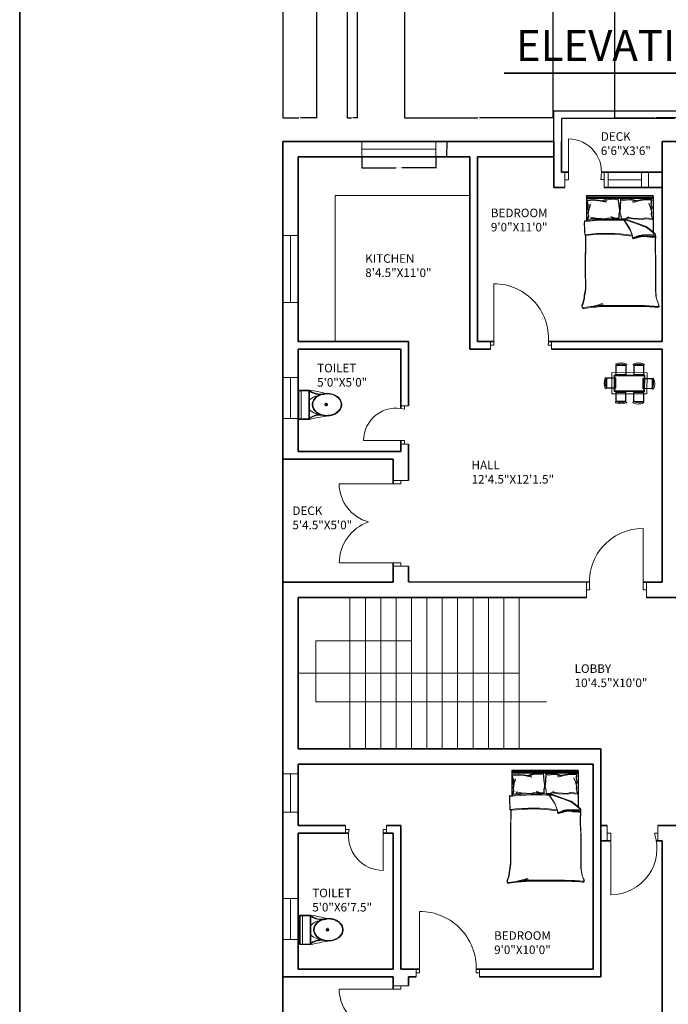
# Model space of a CAD drawing. Units: inches. Extents: x 2250 to 3629, y 982 to 2740.
# Tile 3 of 12: x 2250 to 2629, y 1543 to 2119. Entities that reach past the tile are written whole.
import ezdxf

# ---------------------------------------------------------------- set-up
doc = ezdxf.new("R2010")
doc.units = ezdxf.units.IN
for name, color, linetype, lineweight in [('A-ANNO-DIMS', 2, 'Continuous', 18), ('A-ANNO-TITL', 7, 'Continuous', 35), ('A-ANNO-TTLB', 7, 'Continuous', 35), ('A-AREA-IDEN', 7, 'Continuous', 18), ('A-DOOR', 3, 'Continuous', 18), ('A-FLOR-DECK', 7, 'Continuous', 25), ('A-FLOR-FIXT', 9, 'Continuous', 18), ('A-FLOR-STRS', 7, 'Continuous', 18), ('A-FURN', 8, 'Continuous', 13), ('A-GLAZ', 4, 'Continuous', 18), ('A-WALL', 7, 'Continuous', 35)]:
    doc.layers.add(name, color=color, linetype=linetype, lineweight=lineweight)
doc.styles.get("Standard").update_dxf_attribs({"font": 'arial.ttf'})
doc.dimstyles.get("Standard").update_dxf_attribs({"dimtxt": 0.18, "dimasz": 0.18, "dimexe": 0.18, "dimexo": 0.0625, "dimgap": 0.09, "dimtad": 0, "dimtih": 1, "dimtoh": 1, "dimdec": 4, "dimzin": 0, "dimdsep": 46, "dimtxsty": 'Standard', "dimcen": 0.09, "dimadec": 0, "dimazin": 0, "dimtfac": 1, "dimtdec": 4, "dimtofl": 0, "dimtmove": 0, "dimatfit": 3, "dimfxl": 1, "dimtolj": 1, "dimtzin": 0, "dimarcsym": 0})

# ---------------------------------------------------------------- blocks, each defined once
blk = doc.blocks.new('A$C31115884')
for p, q in [((258, 466), (258, 523)), ((283, 498), (223, 498)), ((0, 200), (0, 0)), ((520, 200), (0, 200)), ((10, 190), (10, 10)), ((510, 190), (10, 190)), ((510, 10), (510, 190)), ((520, 0), (520, 200)), ((510, 54), (0, 54)), ((10, 10), (510, 10)), ((0, 0), (520, 0))]:
    blk.add_line(p, q)
blk.add_circle((256, 496), 23.6)
for centre, radius, start, end in [((2778, -205), 2807, 165.4549, 171.7133), ((-295, 403), 365, 324.2091, 9.3499), ((-295, 403), 375, 324.2091, 9.3499), ((384, 406), 293, 190.2774, 224.1564), ((139, 406), 293, 315.8436, 2.6563), ((806, 403), 375, 179.2036, 215.7909), ((806, 403), 365, 170.6501, 215.7909), ((3237, 905), 2807, 188.2867, 194.5451)]:
    blk.add_arc(centre, radius, start, end)
blk.add_ellipse((256, 510), major_axis=(0, -261), ratio=0.772727)
blk.add_open_spline([(256, 259), (263, 259), (270, 260), (288, 262), (299, 265), (320, 273), (330, 278), (350, 291), (360, 299), (378, 316), (386, 326), (402, 347), (409, 358), (421, 383), (427, 395), (436, 422), (440, 436), (445, 465), (447, 480), (448, 509), (448, 524), (445, 553), (443, 568), (436, 596), (432, 610), (422, 636), (416, 649), (402, 672), (395, 683), (379, 703), (370, 712), (351, 728), (341, 735), (321, 746), (310, 751), (289, 757), (278, 759), (256, 761), (245, 761), (223, 757), (212, 754), (191, 746), (181, 741), (161, 728), (151, 720), (133, 703), (125, 693), (110, 672), (103, 660), (90, 636), (85, 623), (76, 596), (72, 582), (67, 553), (66, 538), (64, 509), (65, 494), (68, 465), (70, 450), (77, 422), (81, 408), (91, 382), (97, 370), (111, 346), (118, 335), (135, 316), (144, 307), (162, 291), (172, 284), (193, 273), (203, 269), (225, 262), (236, 260), (250, 259), (253, 259), (256, 259)], degree=3, knots=[0, 0, 0, 0, 0.110105, 0.110105, 0.285049, 0.285049, 0.459994, 0.459994, 0.634938, 0.634938, 0.809882, 0.809882, 0.984827, 0.984827, 1.159771, 1.159771, 1.334715, 1.334715, 1.50966, 1.50966, 1.684604, 1.684604, 1.859549, 1.859549, 2.034493, 2.034493, 2.209437, 2.209437, 2.384382, 2.384382, 2.559326, 2.559326, 2.73427, 2.73427, 2.909215, 2.909215, 3.084159, 3.084159, 3.259103, 3.259103, 3.434048, 3.434048, 3.608992, 3.608992, 3.783936, 3.783936, 3.958881, 3.958881, 4.133825, 4.133825, 4.30877, 4.30877, 4.483714, 4.483714, 4.658658, 4.658658, 4.833603, 4.833603, 5.008547, 5.008547, 5.183491, 5.183491, 5.358436, 5.358436, 5.53338, 5.53338, 5.708324, 5.708324, 5.883269, 5.883269, 6.058213, 6.058213, 6.233158, 6.233158, 6.283185, 6.283185, 6.283185, 6.283185])
blk = doc.blocks.new('DR-36-BED-NW')
for p, q in [((2, 2.25), (2, 38.25)), ((0, 4.5), (0, 0)), ((0, 0), (0, 2.25)), ((0, 2.25), (2, 2.25)), ((35.76, 2.25), (33.76, 2.25)), ((35.76, 4.5), (35.76, 0)), ((35.76, 0), (35.76, 2.25))]:
    blk.add_line(p, q)
blk.add_arc((2, 6.24), 32.01, 352.83756, 90)
blk = doc.blocks.new('DR-24-DECK-NW')
for p, q in [((2, 4.5), (2, 28.5)), ((0, 9), (0, 0)), ((22.88, 0), (22.88, 9)), ((22.88, 9), (22.88, 4.79)), ((0, 0), (0, 4.5)), ((0, 4.5), (2, 4.5)), ((22.88, 4.79), (20.88, 4.79))]:
    blk.add_line(p, q)
blk.add_arc((2, 9.13), 19.37, 347.05433, 90)
blk = doc.blocks.new('DR-72-DECK-WEST-N')
for p, q in [((36, 48.33), (0, 48.33)), ((31.5, 50.33), (40.5, 50.33)), ((40.5, 50.33), (36, 50.33)), ((36, 50.33), (36, 48.33)), ((36, 2), (0, 2)), ((36, 0), (36, 2)), ((31.5, 0), (40.5, 0)), ((40.5, 0), (36, 0))]:
    blk.add_line(p, q)
for centre, radius, start, end in [((23.09, 48.33), 23.09, 180, 255.18417), ((25.75, 1.72), 25.76, 109.42773, 179.37341)]:
    blk.add_arc(centre, radius, start, end)
blk = doc.blocks.new('DR-24-BATH-NW')
for p, q in [((21.75, 22.45), (26.25, 22.45)), ((26.25, 22.45), (24, 22.45)), ((24, 22.45), (24, 20.45)), ((24, 2), (0, 2)), ((24, 0), (24, 2)), ((21.75, 0), (26.25, 0)), ((26.25, 0), (24, 0))]:
    blk.add_line(p, q)
blk.add_arc((19.09, 2), 19.09, 75.08916, 180)
blk = doc.blocks.new('DR-72-DECK-WEST-S')
for p, q in [((31.5, 47.46), (40.5, 47.46)), ((40.5, 47.46), (36, 47.46)), ((36, 47.46), (36, 45.46)), ((36, 45.46), (0, 45.46)), ((36, 2), (0, 2)), ((36, 0), (36, 2)), ((31.5, 0), (40.5, 0)), ((40.5, 0), (36, 0))]:
    blk.add_line(p, q)
for centre, radius, start, end in [((22.88, 45.46), 22.88, 180, 254.62165), ((25.61, -0.82), 25.77, 109.96423, 173.71154)]:
    blk.add_arc(centre, radius, start, end)
blk = doc.blocks.new('DR-24-BATH-WEST')
for p, q in [((0, 26.25), (0, 21.75)), ((0, 21.75), (0, 24)), ((0, 24), (2, 24)), ((23.91, 24), (21.91, 24)), ((21.91, 24), (21.91, 0)), ((23.91, 21.75), (23.91, 26.25)), ((23.91, 26.25), (23.91, 24))]:
    blk.add_line(p, q)
blk.add_arc((21.91, 20.26), 20.25, 169.34509, 270)
blk = doc.blocks.new('DR-36-BED-WEST')
for p, q in [((2, 2.25), (2, 38.25)), ((0, 4.5), (0, 0)), ((0, 0), (0, 2.25)), ((0, 2.25), (2, 2.25)), ((37.11, 2.25), (35.11, 2.25)), ((37.11, 4.5), (37.11, 0)), ((37.11, 0), (37.11, 2.25))]:
    blk.add_line(p, q)
blk.add_arc((2, 5.02), 33.23, 355.21404, 90)
blk = doc.blocks.new('DR-36-ENTRY-SW')
for p, q in [((0, 40.5), (0, 31.5)), ((29.54, 31.5), (29.54, 40.5)), ((0, 31.5), (0, 36)), ((0, 36), (2, 36)), ((2, 36), (2, 0)), ((29.54, 36), (27.54, 36))]:
    blk.add_line(p, q)
blk.add_arc((2, 27.06), 27.06, 270, 19.28442)
blk = doc.blocks.new('DR-36-ENTRY-NW')
for p, q in [((33.05, 4.5), (33.05, 40.5)), ((0, 9.04), (0, 0)), ((35.05, 9.01), (35.05, 0)), ((0, 0), (0, 4.52)), ((0, 4.52), (2, 4.52)), ((35.05, 4.5), (33.05, 4.5)), ((35.05, 0), (35.05, 4.5))]:
    blk.add_line(p, q)
blk.add_arc((33.05, 9.12), 31.39, 90, 188.41497)
blk = doc.blocks.new('WIN-DECK-NW')
for p, q in [((0.07, 4.5), (0.07, 9)), ((0.07, 9), (0.07, 1.12)), ((19.52, 9), (19.52, 0)), ((0.07, 1.12), (0, 0)), ((19.52, 4.5), (0.07, 4.5)), ((19.52, 0), (19.52, 4.5))]:
    blk.add_line(p, q)
blk = doc.blocks.new('WIN-KITCHEN-NW-A')
for p, q in [((0, 9), (0, 0)), ((43.24, 4.5), (43.24, 9)), ((43.24, 9), (43.24, 0)), ((0, 4.5), (43.24, 4.5))]:
    blk.add_line(p, q)
blk = doc.blocks.new('WIN-KITCHEN-NW-B')
for p, q in [((0, 39.2), (9, 39.2)), ((4.5, 0), (4.5, 39.2)), ((9, 0), (0, 0)), ((0, 0), (4.5, 0))]:
    blk.add_line(p, q)
blk = doc.blocks.new('WIN-24-BATH-NW')
for p, q in [((9, 24), (0, 24)), ((0, 24), (4.5, 24)), ((4.5, 24), (4.5, 0)), ((9, 0), (0, 0)), ((4.5, 0), (9, 0))]:
    blk.add_line(p, q)
blk = doc.blocks.new('WIN-BED-WEST')
for p, q in [((9, 22.49), (0, 22.49)), ((0, 22.49), (4.5, 22.49)), ((4.5, 22.49), (4.5, 0)), ((4.5, 0), (0, 0)), ((0, 0), (9, 0))]:
    blk.add_line(p, q)
blk = doc.blocks.new('BED-WITH-PILLOWS')
for p, q in [((2.83, 51.56), (2.83, 66.3)), ((2.83, 66.3), (41.74, 66.3)), ((2.83, 65.05), (41.74, 65.05)), ((3.02, 51.04), (3.02, 65.78)), ((3.02, 65.78), (41.92, 65.78)), ((3.02, 64.53), (41.92, 64.53)), ((3.17, 63.59), (6.66, 63.85)), ((3.17, 63.6), (3.64, 61.01)), ((6.66, 63.85), (6.75, 63.84)), ((6.75, 63.84), (9.86, 63.6)), ((9.86, 63.6), (14.33, 62.78)), ((12.09, 63.25), (13.74, 63.84)), ((13.74, 63.84), (16.09, 64.43)), ((13.93, 63.32), (16.28, 63.91)), ((16.09, 64.43), (16.36, 64.43)), ((16.28, 63.91), (16.54, 63.91)), ((16.36, 64.43), (19.98, 64.31)), ((16.54, 63.91), (20.16, 63.79)), ((19.98, 64.31), (21.15, 64.78)), ((20.16, 63.79), (21.34, 64.26)), ((21.15, 64.78), (21.62, 60.43)), ((21.34, 64.26), (21.81, 59.9)), ((22.78, 64.27), (22.58, 59.9)), ((22.96, 63.75), (22.76, 59.38)), ((23.98, 63.88), (22.78, 64.27)), ((24.17, 63.36), (22.96, 63.75)), ((27.59, 64.22), (23.98, 63.88)), ((27.77, 63.7), (24.17, 63.36)), ((27.85, 64.24), (27.59, 64.22)), ((28.03, 63.72), (27.77, 63.7)), ((30.23, 63.8), (27.85, 64.24)), ((30.42, 63.28), (28.03, 63.72)), ((34.12, 63.8), (29.71, 62.7)), ((31.91, 63.31), (30.23, 63.8)), ((37.22, 64.23), (34.12, 63.8)), ((37.4, 63.71), (34.31, 63.28)), ((40.8, 64.22), (36.4, 64.3)), ((36.4, 64.3), (37.22, 64.23)), ((40.98, 63.7), (36.58, 63.78)), ((36.58, 63.78), (37.4, 63.71)), ((40.8, 64.22), (40.49, 61.61)), ((40.98, 63.7), (40.67, 61.09)), ((41.74, 66.3), (41.74, 44.64)), ((41.92, 65.78), (41.92, 44.12)), ((3.64, 61.01), (3.29, 58.89)), ((3.29, 58.89), (3.76, 58.07)), ((3.36, 63.06), (6.85, 63.33)), ((3.36, 63.08), (3.83, 60.49)), ((3.83, 60.49), (3.47, 58.37)), ((3.47, 58.37), (3.95, 57.55)), ((3.64, 56.07), (4.11, 59.01)), ((3.83, 55.55), (4.3, 58.49)), ((4.11, 59.01), (4.94, 61.25)), ((4.3, 58.49), (5.12, 60.73)), ((6.85, 63.33), (6.93, 63.32)), ((6.93, 63.32), (10.04, 63.08)), ((10.04, 63.08), (14.52, 62.26)), ((12.28, 62.73), (13.93, 63.32)), ((21.62, 60.43), (22.09, 57.84)), ((21.81, 59.9), (22.28, 57.32)), ((22.09, 57.84), (22.09, 56.78)), ((22.58, 59.9), (22.27, 57.28)), ((22.76, 59.38), (22.46, 56.76)), ((34.31, 63.28), (29.9, 62.18)), ((32.1, 62.79), (30.42, 63.28)), ((40.14, 59.58), (39.18, 61.76)), ((40.33, 59.06), (39.37, 61.24)), ((40.8, 56.67), (40.14, 59.58)), ((40.98, 56.15), (40.33, 59.06)), ((40.49, 61.61), (40.97, 59.51)), ((40.97, 59.51), (40.55, 58.66)), ((40.67, 61.09), (41.16, 58.99)), ((41.16, 58.99), (40.74, 58.14)), ((3.41, 52.19), (3.88, 54.78)), ((7.56, 52.77), (3.41, 52.19)), ((3.59, 51.66), (4.06, 54.25)), ((7.74, 52.25), (3.59, 51.66)), ((3.88, 54.78), (3.64, 56.07)), ((4.06, 54.25), (3.83, 55.55)), ((5.2, 53.58), (8.48, 53.04)), ((5.38, 53.06), (8.66, 52.52)), ((8.48, 53.04), (7.56, 52.77)), ((8.66, 52.52), (7.74, 52.25)), ((8.48, 53.04), (14.18, 52.69)), ((8.66, 52.52), (14.37, 52.17)), ((14.18, 52.69), (15.78, 53.14)), ((14.37, 52.17), (15.97, 52.62)), ((15.78, 53.14), (19.96, 52.81)), ((15.97, 52.62), (20.14, 52.29)), ((19.62, 53.06), (17.06, 53.95)), ((19.81, 52.54), (17.25, 53.43)), ((21.62, 53.06), (19.62, 53.06)), ((21.81, 52.54), (19.81, 52.54)), ((22.09, 56.78), (21.62, 55.25)), ((21.62, 55.25), (21.62, 53.06)), ((22.28, 56.26), (21.81, 54.73)), ((21.81, 54.73), (21.81, 52.54)), ((22.27, 57.28), (22.34, 56.23)), ((22.28, 57.32), (22.28, 56.26)), ((22.34, 56.23), (22.9, 54.73)), ((22.46, 56.76), (22.52, 55.71)), ((22.52, 55.71), (23.09, 54.21)), ((22.9, 54.73), (23.04, 52.55)), ((23.04, 52.55), (25.03, 52.68)), ((23.09, 54.21), (23.22, 52.03)), ((23.22, 52.03), (25.22, 52.15)), ((24.63, 52.15), (28.05, 46.86)), ((25.03, 52.68), (27.53, 53.72)), ((25.22, 52.15), (27.72, 53.2)), ((33.09, 49.76), (26.3, 52.15)), ((26.51, 53.58), (29.79, 53.04)), ((26.7, 53.06), (29.98, 52.52)), ((29.79, 53.04), (35.5, 52.69)), ((29.98, 52.52), (35.69, 52.17)), ((35.5, 52.69), (37.1, 53.14)), ((35.69, 52.17), (37.28, 52.62)), ((37.1, 53.14), (41.27, 52.81)), ((37.28, 52.62), (41.46, 52.29)), ((40.64, 55.37), (40.8, 56.67)), ((41.27, 52.81), (40.64, 55.37)), ((40.83, 54.85), (40.98, 56.15)), ((41.46, 52.29), (40.83, 54.85)), ((24.82, 51.63), (28.23, 46.34)), ((33.27, 49.24), (26.49, 51.63)), ((28.05, 46.86), (29.43, 43.21)), ((28.23, 46.34), (29.62, 42.69)), ((37.63, 48.12), (33.09, 49.76)), ((37.81, 47.6), (33.27, 49.24)), ((40.02, 46.36), (37.63, 48.12)), ((40.21, 45.84), (37.81, 47.6)), ((43.04, 43.71), (40.02, 46.36)), ((29.43, 43.21), (29.68, 41.57)), ((29.62, 42.69), (29.87, 41.05)), ((29.68, 41.57), (31.7, 42.08)), ((29.87, 41.05), (31.89, 41.56)), ((31.7, 42.08), (33.34, 42.83)), ((31.89, 41.56), (33.53, 42.31)), ((33.34, 42.83), (36.11, 43.21)), ((33.53, 42.31), (36.3, 42.69)), ((36.11, 43.21), (39.27, 43.46)), ((36.3, 42.69), (39.45, 42.94)), ((39.27, 43.46), (41.79, 43.21)), ((39.45, 42.94), (41.97, 42.69)), ((43.23, 43.19), (40.21, 45.84)), ((41.79, 43.21), (43.04, 43.71)), ((41.97, 42.69), (43.23, 43.19)), ((43.1, 42.29), (43.04, 43.71, 3.15)), ((43.29, 41.77), (43.23, 43.19, 3.15)), ((12.26, 1.79), (32.3, 1.79)), ((12.45, 1.27), (32.49, 1.27))]:
    blk.add_line(p, q)
for centre, radius, start, end in [((17.39, -81.91), 134.3, 86.08655, 96.78213), ((69.33, 49.94), 67.82, 178.72178, 185.60397), ((69.52, 49.42), 67.82, 178.72178, 185.60397), ((17.57, -82.43), 134.3, 86.08655, 96.78213), ((14.46, -60.96), 105.04, 81.78449, 96.90062), ((14.64, -61.48), 105.04, 81.78449, 96.90062), ((-136.21, 40.92), 138.49, 358.4762, 1.00819), ((-136.02, 40.4), 138.49, 358.4762, 1.00819), ((29.83, 41.52), 0.15, 160.24637, 271.13765), ((25.36, 65.1), 24.14, 280.66171, 289.88058), ((30.01, 41), 0.15, 160.24637, 271.13765), ((25.55, 64.58), 24.14, 280.66171, 289.88058), ((35.61, 37.76), 5.07, 78.6608, 113.73842), ((35.8, 37.23), 5.07, 78.6608, 113.73842), ((41.79, 71.72), 29.46, 259.87628, 272.56571), ((41.97, 71.2), 29.46, 259.87628, 272.56571), ((148.38, 36.74), 105.43, 176.97912, 183.83645), ((148.57, 36.22), 105.43, 176.97912, 183.83645), ((394.7, 25.1), 392.65, 178.22771, 181.71854), ((394.88, 24.58), 392.65, 178.22771, 181.71854), ((-3670.6, 11.09), 3713.84, 0.00217, 0.28689), ((-3670.41, 10.57), 3713.84, 0.00217, 0.28689), ((-21.9, 13.78), 24.13, 346.06484, 358.91125), ((-21.71, 13.26), 24.13, 346.06484, 358.91125), ((-17.63, 9.09), 19.18, 337.97508, 356.652), ((-17.45, 8.57), 19.18, 337.97508, 356.652), ((62, 10.4), 18.78, 177.47136, 206.46809), ((62.19, 9.88), 18.78, 177.47136, 206.46809), ((0.89, 1.4), 0.887, 146.17358, 293.47814), ((1.07, 0.88), 0.887, 146.17358, 293.47814), ((17.44, -97.2), 99.12, 92.99578, 99.40907), ((17.63, -97.72), 99.12, 92.99578, 99.40907), ((-14.02, 85.61), 86.67, 283.38322, 287.70533), ((-13.83, 85.09), 86.67, 283.38322, 287.70533), ((33.5, -106.51), 108.31, 84.4998, 90.63509), ((33.69, -107.03), 108.31, 84.4998, 90.63509), ((44.3, 2.09), 0.897, 242.65876, 356.02002), ((44.48, 1.57), 0.897, 242.65876, 356.02002)]:
    blk.add_arc(centre, radius, start, end)
blk = doc.blocks.new('DINING-SET-6')
for points in [[(7.06, 22.9, -0.175809), (12.68, 22.86, 0.578392), (13.1, 23.32, 0.214524), (6.77, 23.41, 0.552014), (7.06, 22.9, -0.065079)], [(10.61, 22.67), (10.61, 23.33, -0.064759)], [(17.4, 22.86, -0.578392), (16.98, 23.32, -0.214524), (23.31, 23.41, -0.552014), (23.02, 22.9, 0.175809), (17.4, 22.86)], [(19.47, 22.67), (19.47, 23.33, 0.064759)], [(12.44, 22.67), (7.23, 22.67, 0.414214), (6.86, 22.31), (6.86, 17.52, 0.414214), (7.23, 17.15), (12.44, 17.15, 0.414214), (12.8, 17.52), (12.8, 22.31, 0.414214), (12.44, 22.67)], [(22.85, 22.67, -0.414214), (23.22, 22.31), (23.22, 17.52, -0.414214), (22.85, 17.15), (17.64, 17.15, -0.414214), (17.28, 17.52), (17.28, 22.31, -0.414214), (17.64, 22.67), (22.85, 22.67)], [(1.19, 9.34, -0.578392), (0.72, 8.92, -0.214524), (0.64, 15.25, -0.552014), (1.15, 14.96, 0.175809), (1.19, 9.34)], [(1.37, 14.79, -0.414214), (1.74, 15.16), (6.53, 15.16, -0.414214), (6.89, 14.79), (6.89, 9.58, -0.414214), (6.53, 9.22), (1.74, 9.22, -0.414214), (1.37, 9.58), (1.37, 14.79)], [(28.21, 14.61, 0.414214), (27.85, 14.98), (23.05, 14.98, 0.414214), (22.69, 14.61), (22.69, 9.4, 0.414214), (23.05, 9.04), (27.85, 9.04, 0.414214), (28.21, 9.4), (28.21, 14.61)], [(28.44, 14.78, -0.175809), (28.39, 9.16, 0.578392), (28.86, 8.74, 0.214524), (28.95, 15.08, 0.552014), (28.44, 14.78, -0.065079)], [(1.37, 11.41), (0.71, 11.41, 0.064759)], [(12.44, 1.37), (7.23, 1.37, -0.414214), (6.86, 1.74), (6.86, 6.53, -0.414214), (7.23, 6.89), (12.44, 6.89, -0.414214), (12.8, 6.53), (12.8, 1.74, -0.414214), (12.44, 1.37)], [(22.85, 1.37, 0.414214), (23.22, 1.74), (23.22, 6.53, 0.414214), (22.85, 6.89), (17.64, 6.89, 0.414214), (17.28, 6.53), (17.28, 1.74, 0.414214), (17.64, 1.37), (22.85, 1.37)], [(28.21, 11.23), (28.87, 11.23, -0.064759)], [(12.68, 1.19, -0.578392), (13.1, 0.72, -0.214524), (6.77, 0.64, -0.552014), (7.06, 1.15, 0.175809), (12.68, 1.19)], [(10.61, 1.37), (10.61, 0.71, 0.064759)], [(23.02, 1.15, -0.175809), (17.4, 1.19, 0.578392), (16.98, 0.72, 0.214524), (23.31, 0.64, 0.552014), (23.02, 1.15, -0.065079)], [(19.47, 1.37), (19.47, 0.71, -0.064759)]]:
    blk.add_lwpolyline(points, format="xyb")
for points in [[(9.15, 23.35), (9.15, 22.67)], [(20.93, 23.35), (20.93, 22.67)], [(0.7, 12.87), (1.37, 12.87)], [(28.88, 12.69), (28.21, 12.69)], [(9.15, 0.7), (9.15, 1.37)], [(20.93, 0.7), (20.93, 1.37)]]:
    blk.add_lwpolyline(points)
for points in [[(4.51, 18.27), (25.12, 18.27), (25.12, 5.91), (4.51, 5.91)], [(5.89, 16.9), (23.75, 16.9), (23.75, 7.28), (5.89, 7.28)], [(6.3, 16.49), (23.34, 16.49), (23.34, 7.69), (6.3, 7.69)]]:
    blk.add_lwpolyline(points, close=True)
for points in [[(7.23, 22.51), (12.27, 22.51, -0.414214), (12.64, 22.15), (12.64, 17.68, -0.414214), (12.27, 17.32), (7.23, 17.32, -0.512069), (7.03, 17.68), (7.03, 22.15, -0.512069)], [(22.85, 22.51), (17.81, 22.51, 0.414214), (17.44, 22.15), (17.44, 17.68, 0.414214), (17.81, 17.32), (22.85, 17.32, 0.512069), (23.05, 17.68), (23.05, 22.15, 0.512069)], [(1.54, 14.79), (1.54, 9.75, 0.414214), (1.9, 9.38), (6.37, 9.38, 0.414214), (6.73, 9.75), (6.73, 14.79, 0.512069), (6.37, 14.99), (1.9, 14.99, 0.512069)], [(28.05, 14.61), (28.05, 9.57, -0.414214), (27.68, 9.2), (23.22, 9.2, -0.414214), (22.85, 9.57), (22.85, 14.61, -0.512069), (23.22, 14.81), (27.68, 14.81, -0.512069)], [(7.23, 1.54), (12.27, 1.54, 0.414214), (12.64, 1.9), (12.64, 6.36, 0.414214), (12.27, 6.73), (7.23, 6.73, 0.512069), (7.03, 6.36), (7.03, 1.9, 0.512069)], [(22.85, 1.54), (17.81, 1.54, -0.414214), (17.44, 1.9), (17.44, 6.36, -0.414214), (17.81, 6.73), (22.85, 6.73, -0.512069), (23.05, 6.36), (23.05, 1.9, -0.512069)]]:
    blk.add_lwpolyline(points, format="xyb", close=True)
blk = doc.blocks.new('STAIR-RETURN-FLIGHT')
for p, q in [((30.31, 88.5), (30.31, 0)), ((39.31, 88.5), (39.31, 0)), ((48.31, 88.5), (48.31, 0)), ((57.31, 88.5), (57.31, 0)), ((66.31, 88.5), (66.31, 0)), ((75.31, 88.5), (75.31, 0)), ((84.31, 88.5), (84.31, 0)), ((93.31, 88.5), (93.31, 0)), ((102.31, 88.5), (102.31, 0)), ((111.31, 88.5), (111.31, 0)), ((120.31, 88.5), (120.31, 0)), ((129.31, 44.25), (129.31, 88.5)), ((129.31, 88.5), (129.31, 0)), ((10.42, 27.46), (10.42, 63.21)), ((10.42, 63.21), (66.31, 63.21)), ((0, 44.25), (129.31, 44.25)), ((145.28, 27.46), (10.42, 27.46))]:
    blk.add_line(p, q)
blk = doc.blocks.new('*D87')
at = {"layer": 'A-ANNO-DIMS', "color": 0, "lineweight": -2, "transparency": 16777216}
for p, q in [((2449.89, 2038.67), (2449.89, 2032.07)), ((2493.14, 2038.67), (2493.14, 2032.07)), ((2450.07, 2032.25), (2469.82, 2032.25)), ((2492.96, 2032.25), (2473.21, 2032.25))]:
    blk.add_line(p, q, dxfattribs=at)
at = {"layer": 'A-ANNO-DIMS', "color": 0, "transparency": 16777216}
for points in [[(2450.07, 2032.28), (2450.07, 2032.22), (2449.89, 2032.25)], [(2492.96, 2032.28), (2492.96, 2032.22), (2493.14, 2032.25)]]:
    blk.add_solid(points, dxfattribs=at)
at = {"layer": 'Defpoints', "color": 0, "transparency": 16777216}
for p in [(2449.89, 2038.74), (2493.14, 2038.74), (2493.14, 2032.25)]:
    blk.add_point(p, dxfattribs=at)
at = {"layer": 'A-ANNO-DIMS', "color": 0, "transparency": 16777216, "insert": (2471.52, 2032.25), "char_height": 0.18, "attachment_point": 5}
blk.add_mtext('\\A1;KITCHEN WINDOW 43 TYP.', dxfattribs=at)
blk = doc.blocks.new('*D88')
at = {"layer": 'A-ANNO-DIMS', "color": 0, "lineweight": -2, "transparency": 16777216}
for p, q in [((2493.2, 2047.74), (2499.8, 2047.74)), ((2499.62, 2047.56), (2499.62, 2043.42)), ((2499.62, 2038.92), (2499.62, 2043.05)), ((2493.2, 2038.74), (2499.8, 2038.74))]:
    blk.add_line(p, q, dxfattribs=at)
at = {"layer": 'A-ANNO-DIMS', "color": 0, "transparency": 16777216}
for points in [[(2499.59, 2047.56), (2499.65, 2047.56), (2499.62, 2047.74)], [(2499.59, 2038.92), (2499.65, 2038.92), (2499.62, 2038.74)]]:
    blk.add_solid(points, dxfattribs=at)
at = {"layer": 'Defpoints', "color": 0, "transparency": 16777216}
for p in [(2493.14, 2047.74), (2499.62, 2047.74), (2493.14, 2038.74)]:
    blk.add_point(p, dxfattribs=at)
at = {"layer": 'A-ANNO-DIMS', "color": 0, "transparency": 16777216, "insert": (2499.62, 2043.24), "char_height": 0.18, "attachment_point": 5}
blk.add_mtext('\\A1;9 TYP.', dxfattribs=at)
blk = doc.blocks.new('*D170')
at = {"layer": 'A-ANNO-DIMS', "color": 0, "lineweight": -2, "transparency": 16777216}
for p, q in [((2855.4, 2070.24), (2901.69, 2070.24)), ((2901.51, 2070.06), (2901.51, 1664.67)), ((2901.51, 1258.92), (2901.51, 1664.3)), ((2481.67, 1258.74), (2901.69, 1258.74))]:
    blk.add_line(p, q, dxfattribs=at)
at = {"layer": 'A-ANNO-DIMS', "color": 0, "transparency": 16777216}
for points in [[(2901.48, 2070.06), (2901.54, 2070.06), (2901.51, 2070.24)], [(2901.48, 1258.92), (2901.54, 1258.92), (2901.51, 1258.74)]]:
    blk.add_solid(points, dxfattribs=at)
at = {"layer": 'Defpoints', "color": 0, "transparency": 16777216}
for p in [(2855.34, 2070.24), (2901.51, 2070.24), (2481.61, 1258.74)]:
    blk.add_point(p, dxfattribs=at)
at = {"layer": 'A-ANNO-DIMS', "color": 0, "transparency": 16777216, "insert": (2901.51, 1664.49), "char_height": 0.18, "attachment_point": 5}
blk.add_mtext('\\A1;811.5', dxfattribs=at)
blk = doc.blocks.new('*D181')
at = {"layer": 'A-ANNO-DIMS', "color": 0, "lineweight": -2, "transparency": 16777216}
for p, q in [((2423.28, 2191.64), (2423.28, 2061.34)), ((2403.61, 2131.64), (2403.61, 2061.34)), ((2403.79, 2061.52), (2412.99, 2061.52)), ((2423.1, 2061.52), (2413.9, 2061.52))]:
    blk.add_line(p, q, dxfattribs=at)
at = {"layer": 'A-ANNO-DIMS', "color": 0, "transparency": 16777216}
for points in [[(2403.79, 2061.55), (2403.79, 2061.49), (2403.61, 2061.52)], [(2423.1, 2061.55), (2423.1, 2061.49), (2423.28, 2061.52)]]:
    blk.add_solid(points, dxfattribs=at)
at = {"layer": 'Defpoints', "color": 0, "transparency": 16777216}
for p in [(2423.28, 2191.7), (2403.61, 2131.7), (2423.28, 2061.52)]:
    blk.add_point(p, dxfattribs=at)
at = {"layer": 'A-ANNO-DIMS', "color": 0, "transparency": 16777216, "insert": (2413.44, 2061.52), "char_height": 0.18, "attachment_point": 5}
blk.add_mtext('\\A1;19.674', dxfattribs=at)
blk = doc.blocks.new('*D182')
at = {"layer": 'A-ANNO-DIMS', "color": 0, "lineweight": -2, "transparency": 16777216}
for p, q in [((2441.33, 2191.64), (2441.33, 2061.34)), ((2447.11, 2191.64), (2447.11, 2061.34)), ((2441.51, 2061.52), (2443.84, 2061.52)), ((2446.93, 2061.52), (2444.59, 2061.52))]:
    blk.add_line(p, q, dxfattribs=at)
at = {"layer": 'A-ANNO-DIMS', "color": 0, "transparency": 16777216}
for points in [[(2441.51, 2061.55), (2441.51, 2061.49), (2441.33, 2061.52)], [(2446.93, 2061.55), (2446.93, 2061.49), (2447.11, 2061.52)]]:
    blk.add_solid(points, dxfattribs=at)
at = {"layer": 'Defpoints', "color": 0, "transparency": 16777216}
for p in [(2441.33, 2191.7), (2447.11, 2191.7), (2447.11, 2061.52)]:
    blk.add_point(p, dxfattribs=at)
at = {"layer": 'A-ANNO-DIMS', "color": 0, "transparency": 16777216, "insert": (2444.22, 2061.52), "char_height": 0.18, "attachment_point": 5}
blk.add_mtext('\\A1;5.781', dxfattribs=at)
blk = doc.blocks.new('*D183')
at = {"layer": 'A-ANNO-DIMS', "color": 0, "lineweight": -2, "transparency": 16777216}
for p, q in [((2474.74, 2191.64), (2474.74, 2061.34)), ((2561.69, 2173.64), (2561.69, 2061.34)), ((2474.92, 2061.52), (2517.82, 2061.52)), ((2561.51, 2061.52), (2518.61, 2061.52))]:
    blk.add_line(p, q, dxfattribs=at)
at = {"layer": 'A-ANNO-DIMS', "color": 0, "transparency": 16777216}
for points in [[(2474.92, 2061.55), (2474.92, 2061.49), (2474.74, 2061.52)], [(2561.51, 2061.55), (2561.51, 2061.49), (2561.69, 2061.52)]]:
    blk.add_solid(points, dxfattribs=at)
at = {"layer": 'Defpoints', "color": 0, "transparency": 16777216}
for p in [(2474.74, 2191.7), (2561.69, 2173.7), (2561.69, 2061.52)]:
    blk.add_point(p, dxfattribs=at)
at = {"layer": 'A-ANNO-DIMS', "color": 0, "transparency": 16777216, "insert": (2518.22, 2061.52), "char_height": 0.18, "attachment_point": 5}
blk.add_mtext('\\A1;86.94', dxfattribs=at)
blk = doc.blocks.new('*D184')
at = {"layer": 'A-ANNO-DIMS', "color": 0, "lineweight": -2, "transparency": 16777216}
for p, q in [((2645.41, 2191.68), (2645.41, 2061.34)), ((2597.69, 2173.64), (2597.69, 2061.34)), ((2597.87, 2061.52), (2621.08, 2061.52)), ((2645.23, 2061.52), (2622.02, 2061.52))]:
    blk.add_line(p, q, dxfattribs=at)
at = {"layer": 'A-ANNO-DIMS', "color": 0, "transparency": 16777216}
for points in [[(2597.87, 2061.55), (2597.87, 2061.49), (2597.69, 2061.52)], [(2645.23, 2061.55), (2645.23, 2061.49), (2645.41, 2061.52)]]:
    blk.add_solid(points, dxfattribs=at)
at = {"layer": 'Defpoints', "color": 0, "transparency": 16777216}
for p in [(2645.41, 2191.74), (2597.69, 2173.7), (2645.41, 2061.52)]:
    blk.add_point(p, dxfattribs=at)
at = {"layer": 'A-ANNO-DIMS', "color": 0, "transparency": 16777216, "insert": (2621.55, 2061.52), "char_height": 0.18, "attachment_point": 5}
blk.add_mtext('\\A1;47.725', dxfattribs=at)

msp = doc.modelspace()

# ---------------------------------------------------------------- linework, layer by layer
at = {"layer": 'A-ANNO-TITL'}
msp.add_line((2533.1975, 2087.7229), (2686.0181, 2087.7229), dxfattribs=at)
at = {"layer": 'A-ANNO-TTLB'}
msp.add_lwpolyline([(2249.6849, 2739.593), (3629.4532, 2739.593), (3629.4532, 982.3108), (2249.6849, 982.3108)], close=True, dxfattribs=at)
at = {"layer": 'A-FLOR-DECK'}
for p, q in [((2562.1345, 2047.7354), (2562.1345, 2065.7354)), ((2562.1345, 2065.7354), (2637.208, 2065.7354)), ((2632.708, 2061.2354), (2566.6345, 2061.2354)), ((2566.6345, 2061.2354), (2566.6345, 2046.3774))]:
    msp.add_line(p, q, dxfattribs=at)
at = {"layer": 'A-FLOR-FIXT'}
for p, q in [((2434.3344, 1930.7354), (2434.3344, 2016.1232)), ((2434.3344, 2016.1232), (2513.1072, 2016.1232))]:
    msp.add_line(p, q, dxfattribs=at)
at = {"layer": 'A-GLAZ'}
msp.add_line((2617.6296, 2029.7354), (2617.6296, 2020.7354), dxfattribs=at)
at = {"layer": 'A-WALL'}
for p, q in [((2403.6072, 2047.7354), (2403.6072, 1276.7354)), ((2403.6072, 2047.7354), (2562.1345, 2047.7354)), ((2562.1345, 2038.7354), (2562.1345, 2047.7354)), ((2566.6345, 2029.7354), (2566.6345, 2047.7354)), ((2625.6072, 2047.7354), (2625.6072, 1930.7354)), ((2625.6072, 2047.7354), (2778.6072, 2047.7354)), ((2412.6072, 2038.7354), (2513.1072, 2038.7354)), ((2412.6072, 2038.7354), (2412.6072, 1930.7354)), ((2513.1072, 2038.7354), (2513.1072, 1930.7354)), ((2517.6072, 2038.7354), (2517.6072, 1930.7354)), ((2517.6072, 2038.7354), (2562.1345, 2038.7354)), ((2562.1345, 2038.7354), (2562.1345, 2020.7354)), ((2570.7165, 2029.7354), (2566.6345, 2029.7354)), ((2625.6072, 2029.7354), (2590.0847, 2029.7354)), ((2625.6072, 2020.7354), (2625.6072, 2029.7354)), ((2562.1345, 2020.7354), (2568.7165, 2020.7354)), ((2591.5928, 2020.7354), (2625.6072, 2020.7354)), ((2412.6072, 1930.7354), (2462.8572, 1930.7354)), ((2412.6072, 1926.2354), (2462.8572, 1926.2354)), ((2412.6072, 1926.2354), (2412.6072, 1866.2354)), ((2412.6072, 1926.2354), (2472.6072, 1926.2354)), ((2477.1072, 1930.7354), (2462.8572, 1930.7354)), ((2472.6072, 1926.2354), (2472.6072, 1891.4965)), ((2477.1072, 1893.0402), (2477.1072, 1930.7354)), ((2513.1072, 1930.7354), (2513.1072, 1926.2354)), ((2513.1072, 1926.2354), (2525.0488, 1926.2354)), ((2517.6072, 1930.7354), (2527.0488, 1930.7354)), ((2559.0105, 1930.7354), (2625.6072, 1930.7354)), ((2560.8081, 1926.2354), (2625.6072, 1926.2354)), ((2560.8081, 1926.2354), (2625.6072, 1926.2354)), ((2625.6072, 1789.7354), (2625.6072, 1926.2354)), ((2472.6072, 1872.5947), (2472.6072, 1866.2354)), ((2477.1072, 1861.7354), (2477.1072, 1870.5947)), ((2412.6072, 1866.2354), (2462.8572, 1866.2354)), ((2472.6072, 1866.2354), (2462.8572, 1866.2354)), ((2403.6072, 1861.7354), (2462.8572, 1861.7354)), ((2462.8572, 1861.7354), (2468.1072, 1861.7354)), ((2468.1072, 1861.7354), (2468.1072, 1847.3616)), ((2477.1072, 1849.3616), (2477.1072, 1861.7354)), ((2468.1072, 1801.0299), (2468.1072, 1789.7354)), ((2477.1072, 1789.8827), (2477.1072, 1799.0299)), ((2468.1072, 1789.7354), (2403.6072, 1789.7354)), ((2583.0038, 1789.7777), (2477.1072, 1789.8827)), ((2625.6072, 1789.7354), (2614.3928, 1789.7465)), ((2412.6072, 1780.7354), (2477.1072, 1780.7354)), ((2412.6072, 1780.7354), (2412.6072, 1692.2354)), ((2477.1072, 1780.7354), (2581.3416, 1780.7354)), ((2616.3928, 1780.7354), (2625.6072, 1780.7354)), ((2634.7014, 1780.7354), (2625.6072, 1780.7354)), ((2412.6072, 1692.2354), (2585.1072, 1692.2354)), ((2585.1072, 1692.2354), (2589.6072, 1692.2354)), ((2589.6072, 1692.2354), (2589.6072, 1563.2354)), ((2585.1072, 1683.2354), (2412.6072, 1683.2354)), ((2412.6072, 1683.2354), (2412.6072, 1647.2354)), ((2585.1072, 1563.2354), (2585.1072, 1683.2354)), ((2412.6072, 1647.2354), (2440.3572, 1647.2354)), ((2464.263, 1647.2354), (2468.1072, 1647.2354)), ((2468.1072, 1647.2354), (2472.6072, 1647.2354)), ((2472.6072, 1647.2354), (2472.6072, 1618.7354)), ((2589.6072, 1647.2354), (2589.6072, 1638.2354)), ((2593.4516, 1647.2354), (2589.6072, 1647.2354)), ((2647.0484, 1647.2354), (2622.9956, 1647.2354)), ((2412.6072, 1642.7354), (2412.6072, 1563.2354)), ((2442.0632, 1642.7354), (2412.6072, 1642.7354)), ((2468.1072, 1642.7354), (2462.263, 1642.7354)), ((2468.1072, 1563.2354), (2468.1072, 1642.7354)), ((2589.6072, 1638.2354), (2595.4516, 1638.2354)), ((2622.1478, 1638.2354), (2625.6072, 1638.2354)), ((2625.6072, 1638.2354), (2625.6072, 1434.2354)), ((2472.6072, 1563.2354), (2472.6072, 1618.7354)), ((2412.6072, 1563.2354), (2468.1072, 1563.2354)), ((2472.6072, 1563.2354), (2477.1072, 1563.2354)), ((2477.1072, 1563.2354), (2483.5866, 1563.2354)), ((2516.8102, 1563.2354), (2585.1072, 1563.2354)), ((2589.6072, 1563.2354), (2589.6072, 1558.7354)), ((2412.6072, 1558.7354), (2403.6072, 1558.7354)), ((2412.6072, 1558.7354), (2468.1072, 1558.7354)), ((2468.1072, 1558.7354), (2468.1072, 1551.4204)), ((2477.1072, 1553.4204), (2477.1072, 1558.7354)), ((2481.5866, 1558.7354), (2477.1072, 1558.7354)), ((2589.6072, 1558.7354), (2518.6984, 1558.7354))]:
    msp.add_line(p, q, dxfattribs=at)

# ---------------------------------------------------------------- block references
at = {"layer": 'A-DOOR'}
for name, p in [('DR-24-DECK-NW', (2568.717, 2020.735)), ('DR-36-BED-NW', (2525.049, 1926.235)), ('DR-24-BATH-NW', (2450.857, 1870.595)), ('DR-72-DECK-WEST-N', (2436.607, 1799.03)), ('DR-36-ENTRY-NW', (2581.342, 1780.735)), ('DR-24-BATH-WEST', (2440.357, 1620.985)), ('DR-36-ENTRY-SW', (2593.452, 1606.735)), ('DR-36-BED-WEST', (2481.587, 1558.735)), ('DR-72-DECK-WEST-S', (2436.607, 1505.964))]:
    msp.add_blockref(name, p, dxfattribs=at)
at = {"layer": 'A-FLOR-FIXT', "xscale": 0.0330640103915726, "yscale": 0.0330640103915726, "zscale": 0.0330640103915726, "rotation": 269.9999999999999}
for p in [(2412.6072, 1902.1854), (2413.4396, 1594.7225)]:
    msp.add_blockref('A$C31115884', p, dxfattribs=at)
at = {"layer": 'A-FLOR-STRS'}
msp.add_blockref('STAIR-RETURN-FLIGHT', (2412.607, 1692.235), dxfattribs=at)
at = {"layer": 'A-FURN'}
for p in [(2578.511, 1949.878), (2534.7066, 1613.3968)]:
    msp.add_blockref('BED-WITH-PILLOWS', p, dxfattribs=at)
at = {"layer": 'A-FURN', "rotation": 359.5962358253915}
msp.add_blockref('DINING-SET-6', (2591.5318, 1894.1863), dxfattribs=at)
at = {"layer": 'A-GLAZ'}
for name, p in [('WIN-KITCHEN-NW-A', (2449.895, 2038.735)), ('WIN-DECK-NW', (2593.871, 2020.735)), ('WIN-KITCHEN-NW-B', (2403.607, 1953.486)), ('WIN-24-BATH-NW', (2403.607, 1885.572)), ('WIN-BED-WEST', (2403.607, 1655.016))]:
    msp.add_blockref(name, p, dxfattribs=at)
at = {"layer": 'A-GLAZ', "rotation": 180}
msp.add_blockref('WIN-24-BATH-NW', (2412.6074, 1604.5739), dxfattribs=at)

# ---------------------------------------------------------------- texts
at = {"layer": 'A-ANNO-TITL', "insert": (2540.0175, 2112.9477), "char_height": 18, "attachment_point": 1}
msp.add_mtext_dynamic_manual_height_columns('ELEVATION', width=205.216526, gutter_width=12.5, heights=[0], dxfattribs=at)
at = {"layer": 'A-AREA-IDEN', "char_height": 5, "attachment_point": 1}
for s, width, insert in [('DECK\\P6\'6"X3\'6"', 73.673866, (2589.6665, 2053.1628)), ('BEDROOM\\P9\'0"X11\'0"', 111.483335, (2525.3616, 2008.4337)), ('KITCHEN\\P8\'4.5"X11\'0"', 145.2909, (2451.85, 1981.728)), ('TOILET\\P5\'0"X5\'0"', 97.52064, (2423.7036, 1917.5771)), ('HALL\\P12\'4.5"X12\'1.5"', 136.888587, (2514.0612, 1860.8031)), ('DECK\\P5\'4.5"X5\'0"', 84.223367, (2409.2298, 1834.0556)), ('LOBBY\\P10\'4.5"X10\'0"', 217.987734, (2574.364, 1741.6377)), ('TOILET\\P5\'0"X6\'7.5"', 97.354189, (2420.8306, 1610.2807)), ('BEDROOM\\P9\'0"X10\'0"', 98.33221, (2527.275, 1585.3523))]:
    msp.add_mtext_dynamic_manual_height_columns(s, width=width, gutter_width=12.5, heights=[0], dxfattribs=dict(at, insert=insert))

# ---------------------------------------------------------------- dimensions: what is measured, and where the dimension line sits
at = {"layer": 'A-ANNO-DIMS'}
for base, p1, p2, override, picture, middle in [((2423.2815, 2061.5229), (2403.6072, 2131.6999), (2423.2815, 2191.6999), {"dimdec": 3, "dimlfac": 1, "dimrnd": 0, "dimzin": 0, "dimdsep": 46, "dimlunit": 2}, '*D181', (2413.4444, 2061.5229)), ((2447.1072, 2061.5229), (2441.3258, 2191.6999), (2447.1072, 2191.6999), {"dimdec": 3, "dimlfac": 1, "dimrnd": 0, "dimzin": 0, "dimdsep": 46, "dimlunit": 2}, '*D182', (2444.2165, 2061.5229)), ((2561.6892, 2061.5229), (2474.7443, 2191.6999), (2561.6892, 2173.6999), {"dimdec": 2, "dimlfac": 1, "dimrnd": 0, "dimzin": 0, "dimdsep": 46, "dimlunit": 2}, '*D183', (2518.2168, 2061.5229)), ((2645.4141, 2061.5229), (2597.6892, 2173.6999), (2645.4141, 2191.7387), {"dimdec": 3, "dimlfac": 1, "dimrnd": 0, "dimzin": 0, "dimdsep": 46, "dimlunit": 2}, '*D184', (2621.5517, 2061.5229))]:
    dim = msp.add_linear_dim(base=base, p1=p1, p2=p2, dimstyle='Standard', override=override, dxfattribs=at)
    dim.commit()
    dim.dimension.update_dxf_attribs({"geometry": picture, "text_midpoint": middle})
dim = msp.add_linear_dim(base=(2901.5072, 2070.2354), p1=(2481.6072, 1258.7354), p2=(2855.3384, 2070.2354), angle=90, dimstyle='Standard', override={"dimdec": 1, "dimlfac": 1, "dimrnd": 0, "dimzin": 0, "dimdsep": 46, "dimlunit": 2}, dxfattribs=at)
dim.commit()
dim.dimension.update_dxf_attribs({"geometry": '*D170', "text_midpoint": (2901.5072, 1664.4854)})
dim = msp.add_linear_dim(base=(2499.6223, 2047.7354), p1=(2493.1361, 2038.7354), p2=(2493.1361, 2047.7354), angle=90, text='<> TYP.', dimstyle='Standard', override={"dimdec": 0, "dimlfac": 1, "dimrnd": 0, "dimzin": 0, "dimdsep": 46, "dimlunit": 2}, dxfattribs=at)
dim.commit()
dim.dimension.update_dxf_attribs({"geometry": '*D88', "text_midpoint": (2499.6223, 2043.2354)})
dim = msp.add_linear_dim(base=(2493.1361, 2032.2492), p1=(2449.8949, 2038.7354), p2=(2493.1361, 2038.7354), text='KITCHEN WINDOW <> TYP.', dimstyle='Standard', override={"dimdec": 0, "dimlfac": 1, "dimrnd": 0, "dimzin": 0, "dimdsep": 46, "dimlunit": 2}, dxfattribs=at)
dim.commit()
dim.dimension.update_dxf_attribs({"geometry": '*D87', "text_midpoint": (2471.5155, 2032.2492)})

doc.saveas('drawing.dxf')
